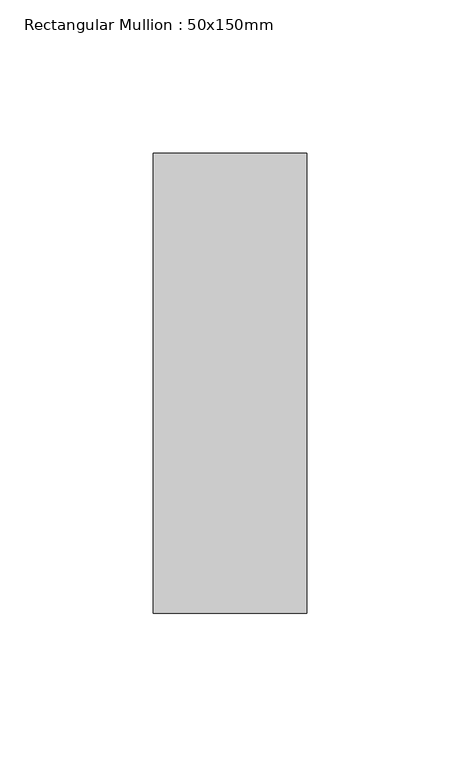
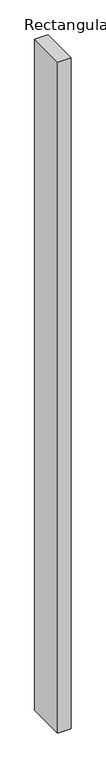
"""IFC4 building model written with IfcOpenShell, lengths in millimetres: member geometry, Rectangular Mullion : 50x150mm."""

from ifc_helpers import new_model, si_unit, frame, origin, place, context, project, spatial, polyline, outline, extrude, source, transform, mapped, element, save


def rectangular_mullion_50x150mm_5671121a(model_context):
    return source(origin(), model_context, "Body", "SweptSolid", [
        extrude(outline(polyline([(0.0, 75.0), (0.0, -75.0), (-50.0, -75.0), (-50.0, 75.0), (0.0, 75.0)])), frame((0.0, 0.0, -2674.95), z_axis=(0.0, 0.0, 1.0), x_axis=(1.0, 0.0, 0.0)), (0.0, 0.0, 1.0), 2674.95),
    ])


if __name__ == "__main__":
    model = new_model("IFC4")
    model_context = context("Model", 3, world=origin())
    ifc_project = project(units=[si_unit("LENGTHUNIT", "METRE", prefix="MILLI")], contexts=[model_context])
    site = spatial("IfcSite", under=ifc_project)
    building = spatial("IfcBuilding", under=site)
    placement = place(None, origin())
    rectangular_mullion_50x150mm_shape = rectangular_mullion_50x150mm_5671121a(model_context)
    element("IfcMember", 1, ObjectType="Rectangular Mullion : 50x150mm", at=placement, inside=building, context=model_context, shape_type="MappedRepresentation", body=[
        mapped(rectangular_mullion_50x150mm_shape, transform((0.0, 0.0, 0.0), x_axis=(1.0, 0.0, 0.0), y_axis=(0.0, 1.0, 0.0), z_axis=(0.0, 0.0, 1.0))),
    ])
    save(model, "model.ifc")

# Revit data of these elements
# Type "Rectangular Mullion : 50x150mm"
#   Keynote = "H11"
#   built-in parameter 1007304 = 0.492126 (stored number, unit not read)
#   built-in parameter 1007301 = 0.082021 (stored number, unit not read)
#   built-in parameter 1007300 = 0.082021 (stored number, unit not read)
# Element 1 (IfcMember, "Rectangular Mullion : 50x150mm")
#   Materials on its faces: "Aluminium"
# Materials
#   "Aluminium": class "Metal", colour RGB 247 247 247, transparency 0, Description = "Aluminium 6061", Cost = 0
